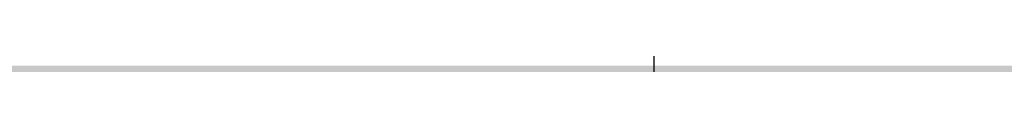
# Model space of a CAD drawing. Units: inches. Extents: x 2083 to 3317, y 1141 to 2115.
# Tile 60 of 256: x 2237.106 to 2238.294, y 1477.763 to 1477.764. Entities that reach past the tile are written whole.
import ezdxf

# ---------------------------------------------------------------- set-up
doc = ezdxf.new("R2010")
doc.units = ezdxf.units.IN
doc.layers.add('A-ANNO-DIMS', color=2, linetype='Continuous', lineweight=18)
doc.layers.add('A-WALL-PATT', color=251, linetype='Continuous', lineweight=13, true_color=0x636466)
doc.styles.get("Standard").update_dxf_attribs({"font": 'arial.ttf'})
doc.dimstyles.new('ISO-25', dxfattribs={"dimtxt": 12, "dimasz": 12, "dimexe": 1.25, "dimexo": 0.625, "dimtad": 1, "dimlunit": 3, "dimtxsty": 'Standard', "dimcen": 2.5, "dimadec": 0, "dimazin": 0, "dimtfac": 1, "dimtmove": 0, "dimatfit": 3, "dimfxl": 1, "dimarcsym": 0})

# ---------------------------------------------------------------- blocks, each defined once
blk = doc.blocks.new('*D30')
at = {"layer": 'A-ANNO-DIMS', "color": 0, "lineweight": -2, "transparency": 16777216}
for p, q in [((2240.0179, 1445.2738), (2240.0179, 1448.0455)), ((2254.3293, 1445.2738), (2254.3293, 1448.0455)), ((2228.0179, 1446.7955), (2216.0179, 1446.7955)), ((2240.0179, 1446.7955), (2254.3293, 1446.7955)), ((2266.3293, 1446.7955), (2413.7649, 1446.7955))]:
    blk.add_line(p, q, dxfattribs=at)
at = {"layer": 'A-ANNO-DIMS', "color": 0, "transparency": 16777216}
for points in [[(2228.0179, 1448.7955), (2228.0179, 1444.7955), (2240.0179, 1446.7955)], [(2266.3293, 1448.7955), (2266.3293, 1444.7955), (2254.3293, 1446.7955)]]:
    blk.add_solid(points, dxfattribs=at)
at = {"layer": 'Defpoints', "color": 0, "transparency": 16777216}
for p in [(2254.3293, 1446.7955), (2240.0179, 1444.6488), (2254.3293, 1444.6488)]:
    blk.add_point(p, dxfattribs=at)
at = {"layer": 'A-ANNO-DIMS', "color": 0, "transparency": 16777216, "insert": (2346.0471, 1453.6252), "char_height": 12, "attachment_point": 5}
blk.add_mtext('WC 1\'-2 1/2" TYP.', dxfattribs=at)
blk = doc.blocks.new('*D31')
at = {"layer": 'A-ANNO-DIMS', "color": 0, "lineweight": -2, "transparency": 16777216}
for p, q in [((2237.8711, 1456.6488), (2237.8711, 1541.9152)), ((2239.3929, 1444.6488), (2236.6211, 1444.6488)), ((2237.8711, 1431.5475), (2237.8711, 1444.6488)), ((2239.3929, 1431.5475), (2236.6211, 1431.5475)), ((2237.8711, 1419.5475), (2237.8711, 1407.5475))]:
    blk.add_line(p, q, dxfattribs=at)
at = {"layer": 'A-ANNO-DIMS', "color": 0, "transparency": 16777216}
for points in [[(2235.8711, 1456.6488), (2239.8711, 1456.6488), (2237.8711, 1444.6488)], [(2235.8711, 1419.5475), (2239.8711, 1419.5475), (2237.8711, 1431.5475)]]:
    blk.add_solid(points, dxfattribs=at)
at = {"layer": 'Defpoints', "color": 0, "transparency": 16777216}
for p in [(2237.8711, 1444.6488), (2240.0179, 1444.6488), (2240.0179, 1431.5475)]:
    blk.add_point(p, dxfattribs=at)
at = {"layer": 'A-ANNO-DIMS', "color": 0, "transparency": 16777216, "insert": (2231.2175, 1505.282), "char_height": 12, "attachment_point": 5, "rotation": 90}
blk.add_mtext('1\'-1" TYP.', dxfattribs=at)
blk = doc.blocks.new('*D45')
at = {"layer": 'A-ANNO-DIMS', "color": 0, "lineweight": -2, "transparency": 16777216}
for p, q in [((2235.9598, 1478.3864), (2235.9598, 1531.3614)), ((2418.9598, 1478.3864), (2418.9598, 1531.3614)), ((2247.9598, 1530.1114), (2406.9598, 1530.1114))]:
    blk.add_line(p, q, dxfattribs=at)
at = {"layer": 'A-ANNO-DIMS', "color": 0, "transparency": 16777216}
for points in [[(2247.9598, 1532.1114), (2247.9598, 1528.1114), (2235.9598, 1530.1114)], [(2406.9598, 1532.1114), (2406.9598, 1528.1114), (2418.9598, 1530.1114)]]:
    blk.add_solid(points, dxfattribs=at)
at = {"layer": 'Defpoints', "color": 0, "transparency": 16777216}
for p in [(2418.9598, 1530.1114), (2235.9598, 1477.7614), (2418.9598, 1477.7614)]:
    blk.add_point(p, dxfattribs=at)
at = {"layer": 'A-ANNO-DIMS', "color": 0, "transparency": 16777216, "insert": (2327.4598, 1536.8673), "char_height": 12, "attachment_point": 5}
blk.add_mtext('15\'-3"', dxfattribs=at)
blk = doc.blocks.new('*D62')
at = {"layer": 'A-ANNO-DIMS', "color": 0, "lineweight": -2, "transparency": 16777216}
for p, q in [((2235.9598, 1469.3864), (2235.9598, 1522.3614)), ((2379.9598, 1469.3864), (2379.9598, 1522.3614)), ((2247.9598, 1521.1114), (2367.9598, 1521.1114))]:
    blk.add_line(p, q, dxfattribs=at)
at = {"layer": 'A-ANNO-DIMS', "color": 0, "transparency": 16777216}
for points in [[(2247.9598, 1523.1114), (2247.9598, 1519.1114), (2235.9598, 1521.1114)], [(2367.9598, 1523.1114), (2367.9598, 1519.1114), (2379.9598, 1521.1114)]]:
    blk.add_solid(points, dxfattribs=at)
at = {"layer": 'Defpoints', "color": 0, "transparency": 16777216}
for p in [(2379.9598, 1521.1114), (2235.9598, 1468.7614), (2379.9598, 1468.7614)]:
    blk.add_point(p, dxfattribs=at)
at = {"layer": 'A-ANNO-DIMS', "color": 0, "transparency": 16777216, "insert": (2307.9598, 1527.8632), "char_height": 12, "attachment_point": 5}
blk.add_mtext('12\'-0"', dxfattribs=at)

msp = doc.modelspace()

# ---------------------------------------------------------------- hatches: boundary and pattern name
at = {"layer": 'A-WALL-PATT'}
h = msp.add_hatch(color=256, dxfattribs=at)
h.dxf.hatch_style = 1
h.paths.add_polyline_path([(3126.9598, 2020.7614), (2748.9598, 2020.7614), (2604.9598, 2020.7614), (2226.9598, 2020.7614), (2226.9598, 1702.7614), (2466.9598, 1702.7614), (2466.9598, 1582.7614), (2418.9598, 1582.7614), (2418.9598, 1477.7614), (2226.9598, 1477.7614), (2226.9598, 1263.2614), (2544.9598, 1263.2614), (2544.9598, 1411.7614), (2604.9598, 1411.7614), (2685.9598, 1411.7614), (2685.9598, 1420.7614), (2604.9598, 1420.7614), (2604.9598, 1573.7614), (2604.9598, 1702.7614), (2604.9598, 2011.7614), (2748.9598, 2011.7614), (2748.9598, 1702.7614), (2862.9598, 1702.7614), (2862.9598, 1621.7614), (2871.9598, 1621.7614), (2871.9598, 1702.7614), (2883.9598, 1702.7614), (2883.9598, 1706.9395, -0.026459), (2883.9598, 1711.7614), (2757.9598, 1711.7614), (2757.9598, 1807.7614), (2787.9598, 1807.7614), (2787.9598, 1812.2614), (2757.9598, 1812.2614), (2757.9598, 2011.7614), (2877.9598, 2011.7614), (2877.9598, 1812.2614), (2847.9598, 1812.2614), (2847.9598, 1807.7614), (2889.8357, 1807.7614), (2889.8357, 1812.2614), (2882.4598, 1812.2614), (2882.4598, 2011.7614), (3117.9598, 2011.7614), (3117.9598, 1812.2614), (2937.8357, 1812.2614), (2937.8357, 1807.7614), (2995.7098, 1807.7614), (2995.7098, 1796.1177), (3000.2098, 1796.1177), (3000.2098, 1807.7614), (3117.9598, 1807.7614), (3117.9598, 1711.7614), (3000.2098, 1711.7614), (3000.2098, 1760.1177), (2998.5727, 1760.1177, -0.020711), (2995.7098, 1760.1177), (2995.7098, 1711.7614), (2931.9598, 1711.7614), (2931.9598, 1702.7614), (3126.9598, 1702.7614)])
h.paths.add_polyline_path([(2471.4598, 2011.7614), (2471.4598, 1810.0114), (2462.7169, 1810.0114), (2462.7169, 1805.5114), (2505.9598, 1805.5114), (2505.9598, 1810.0114), (2475.9598, 1810.0114), (2475.9598, 2011.7614), (2595.9598, 2011.7614), (2595.9598, 1810.0114), (2565.9598, 1810.0114), (2565.9598, 1805.5114), (2595.9598, 1805.5114), (2595.9598, 1711.7614), (2235.9598, 1711.7614), (2235.9598, 1805.5114), (2353.7098, 1805.5114), (2353.7098, 1796.0542), (2358.2098, 1796.0542), (2358.2098, 1805.5114), (2414.7169, 1805.5114), (2414.7169, 1810.0114), (2235.9598, 1810.0114), (2235.9598, 2011.7614)], flags=16)
h.paths.add_polyline_path([(2270.2047, 1994.61), (2270.2047, 1970.61), (2246.2047, 1970.61), (2246.2047, 1994.61)], flags=0)
edge = h.paths.add_edge_path(flags=0)
edge.add_ellipse((2332.0274, 1899.7982), major_axis=(-3.043, 3.043), ratio=0.168252, start_angle=-161.3322, end_angle=-156.3071, ccw=False)
edge.add_ellipse((2333.082, 1898.7435), major_axis=(-1.0546, 1.0546), ratio=0.453532, start_angle=-123.371, end_angle=-94.1591)
edge = h.paths.add_edge_path(flags=0)
edge.add_ellipse((2332.0274, 1968.8763), major_axis=(3.043, 3.043), ratio=0.168252, start_angle=18.6678, end_angle=23.6929)
edge.add_spline(control_points=[(2332.9256, 1970.6911), (2332.2268, 1970.3361), (2330.8937, 1969.6589), (2328.4131, 1970.9321), (2327.2039, 1967.7487), (2324.7096, 1969.9556), (2322.5328, 1967.0124), (2320.0128, 1971.2958), (2317.6803, 1968.1578), (2316.0405, 1967.102), (2315.4269, 1966.8096)], knot_values=[0, 0, 0, 0, 2.267059, 4.324559, 6.685584, 8.878641, 11.121502, 14.300359, 17.755284, 19.732645, 19.732645, 19.732645, 19.732645], degree=3, periodic=0)
edge.add_ellipse((2332.0274, 1968.8763), major_axis=(3.043, 3.043), ratio=0.168252, start_angle=18.6678, end_angle=23.6929, ccw=False)
edge.add_ellipse((2333.082, 1969.9309), major_axis=(1.0546, 1.0546), ratio=0.453532, start_angle=56.629, end_angle=85.8409, ccw=False)
edge = h.paths.add_edge_path(flags=0)
edge.add_spline(control_points=[(2296.4283, 1967.9879), (2293.6278, 1965.3363), (2287.7036, 1959.7271), (2299.7439, 1949.9957), (2294.5326, 1935.6685), (2290.5732, 1920.6035), (2293.3941, 1909.9737), (2296.1854, 1904.9665)], knot_values=[0.099185, 0.099185, 0.099185, 0.099185, 0.345301, 0.619822, 0.982653, 1.386093, 1.810555, 1.810555, 1.810555, 1.810555], degree=3, periodic=0)
edge.add_spline(control_points=[(2296.1854, 1904.9665), (2297.3836, 1902.6193), (2298.001, 1901.9493), (2298.553, 1901.4682)], knot_values=[0.006246, 0.006246, 0.006246, 0.006246, 0.055476, 0.055476, 0.055476, 0.055476], degree=3, periodic=0)
edge.add_spline(control_points=[(2298.553, 1901.4682), (2297.2586, 1900.9232), (2295.2253, 1900.2321), (2293.0602, 1900.6142), (2292.1014, 1900.7884), (2292.0896, 1900.7906)], knot_values=[0.312835, 0.312835, 0.312835, 0.312835, 0.40178, 0.474987, 0.475903, 0.475903, 0.475903, 0.475903], degree=3, periodic=0)
edge.add_arc((2292.7936, 1904.6641), 3.937, 215.4209, 259.6982, ccw=False)
edge.add_spline(control_points=[(2289.5853, 1902.3823), (2289.4767, 1902.5351), (2289.3685, 1902.688), (2289.2609, 1902.8412)], knot_values=[0.102872, 0.102872, 0.102872, 0.102872, 0.116896, 0.116896, 0.116896, 0.116896], degree=3, periodic=0)
edge.add_spline(control_points=[(2289.2609, 1902.8412), (2288.6866, 1902.5502), (2287.64, 1902.0199), (2285.8813, 1901.874), (2283.853, 1901.5044), (2281.72, 1899.7105), (2278.467, 1899.4929), (2276.1571, 1901.8832), (2272.259, 1899.8041), (2267.7776, 1901.8432), (2262.2439, 1900.184), (2257.4149, 1901.7821), (2254.3184, 1900.7261), (2253.1783, 1900.3373)], knot_values=[0, 0, 0, 0, 1.907977, 3.477176, 5.261074, 7.972851, 11.680248, 13.717921, 16.939592, 22.789562, 27.502503, 33.595215, 37.145618, 37.145618, 37.145618, 37.145618], degree=3, periodic=0)
edge.add_line((2253.1783, 1900.3373), (2250.2442, 1902.8412))
edge.add_line((2250.2442, 1902.8412), (2250.2442, 1965.8333))
edge.add_line((2250.2442, 1965.8333), (2253.1783, 1968.3371))
edge.add_spline(control_points=[(2253.1783, 1968.3371), (2254.3184, 1967.9483), (2257.4149, 1966.8924), (2262.2439, 1968.4904), (2267.7776, 1966.8313), (2271.5267, 1968.5372), (2273.8759, 1967.8283), (2274.2067, 1967.7276)], knot_values=[0, 0, 0, 0, 0.09018, 0.244935, 0.364644, 0.513233, 0.537855, 0.537855, 0.537855, 0.537855], degree=3, periodic=0)
edge.add_arc((2274.3529, 1963.7933), 3.937, 72.0511, 92.1279, ccw=False)
edge.add_arc((2281.2969, 1985.23), 18.5963, 252.05113, 288.56572)
edge.add_arc((2292.3167, 1956.0289), 12.6461, 71.02679, 113.77822, ccw=False)
edge = h.paths.add_edge_path(flags=0)
edge.add_spline(control_points=[(2274.8994, 1951.8562), (2275.0662, 1951.6166), (2275.2327, 1951.3766), (2275.398, 1951.1359)], knot_values=[1.409916, 1.409916, 1.409916, 1.409916, 1.43159, 1.43159, 1.43159, 1.43159], degree=3, periodic=0)
edge.add_spline(control_points=[(2275.398, 1951.1359), (2275.7921, 1950.5619), (2276.1792, 1949.9838), (2276.5455, 1949.3971)], knot_values=[1.358238, 1.358238, 1.358238, 1.358238, 1.409916, 1.409916, 1.409916, 1.409916], degree=3, periodic=0)
edge.add_line((2276.5455, 1949.3971), (2277.4373, 1947.8622))
edge.add_spline(control_points=[(2277.4373, 1947.8622), (2276.3038, 1945.6731), (2274.6397, 1942.4269), (2274.6316, 1938.0939), (2272.7991, 1930.8515), (2274.3564, 1943.897), (2275.9477, 1947.9234), (2276.5455, 1949.3971)], knot_values=[0.005632, 0.005632, 0.005632, 0.005632, 0.186014, 0.266002, 0.357087, 0.59639, 0.739732, 0.739732, 0.739732, 0.739732], degree=3, periodic=0)
edge.add_spline(control_points=[(2276.5455, 1949.3971), (2276.1792, 1949.9838), (2275.7921, 1950.5619), (2275.398, 1951.1359)], knot_values=[1.358238, 1.358238, 1.358238, 1.358238, 1.409916, 1.409916, 1.409916, 1.409916], degree=3, periodic=0)
edge.add_spline(control_points=[(2275.398, 1951.1359), (2274.9425, 1950.0805), (2274.2078, 1948.0253), (2273.9346, 1944.8515), (2272.4685, 1937.6275), (2273.4662, 1945.6965), (2274.7006, 1951.0595), (2274.8994, 1951.8562)], knot_values=[0.104364, 0.104364, 0.104364, 0.104364, 0.189636, 0.269624, 0.36071, 0.600013, 0.644622, 0.644622, 0.644622, 0.644622], degree=3, periodic=0)
h.paths.add_polyline_path([(2269.1675, 1963.1276, -0.357527), (2268.1706, 1960.9764, -0.092561), (2268.1706, 1939.4363, -0.357527), (2269.1675, 1937.2851, -0.357527), (2267.0163, 1938.282, -0.164785), (2254.6856, 1938.282, -0.357527), (2252.5344, 1937.2851, -0.357527), (2253.5313, 1939.4363, -0.092561), (2253.5313, 1960.9764, -0.357527), (2252.5344, 1963.1276, -0.357527), (2254.6856, 1962.1307, -0.164785), (2267.0163, 1962.1307, -0.357527)], flags=0)
h.paths.add_polyline_path([(2248.8741, 1967.8018), (2248.8741, 1957.0277), (2249.4578, 1957.0277), (2249.4578, 1911.6468), (2248.8741, 1911.6468), (2248.8741, 1900.8727), (2246.5119, 1900.8727, 0.197327), (2244.1497, 1902.4569), (2244.1497, 1966.2176, 0.197327), (2246.5119, 1967.8018)], flags=0)
h.paths.add_polyline_path([(2269.1675, 1931.3893, -0.357527), (2268.1706, 1929.2381, -0.092561), (2268.1706, 1907.6981, -0.357527), (2269.1675, 1905.5469, -0.357527), (2267.0163, 1906.5438, -0.164785), (2254.6856, 1906.5438, -0.357527), (2252.5344, 1905.5469, -0.357527), (2253.5313, 1907.6981, -0.092561), (2253.5313, 1929.2381, -0.357527), (2252.5344, 1931.3893, -0.357527), (2254.6856, 1930.3925, -0.164785), (2267.0163, 1930.3925, -0.357527)], flags=0)
edge = h.paths.add_edge_path(flags=0)
edge.add_spline(control_points=[(2276.1969, 1906.7237), (2276.1681, 1909.0289), (2276.114, 1913.3719), (2270.5984, 1924.925), (2273.9052, 1919.0128), (2275.9217, 1916.2621), (2275.4746, 1912.4021), (2277.2579, 1910.3806), (2276.696, 1908.225), (2276.6462, 1906.813), (2276.6178, 1906.0084)], knot_values=[0, 0, 0, 0, 8.61026, 16.221274, 18.843057, 23.804898, 27.440828, 29.356102, 31.203478, 33.650687, 33.650687, 33.650687, 33.650687], degree=3, periodic=0)
edge.add_spline(control_points=[(2276.6178, 1906.0084), (2276.6233, 1905.6241), (2276.4977, 1904.6287), (2275.4418, 1903.8547), (2274.9373, 1903.0804), (2274.8591, 1902.8412)], knot_values=[0.156488, 0.156488, 0.156488, 0.156488, 0.184398, 0.231376, 0.250598, 0.250598, 0.250598, 0.250598], degree=3, periodic=0)
edge.add_line((2274.8591, 1902.8412), (2276.506, 1902.8412))
edge.add_spline(control_points=[(2276.506, 1902.8412), (2276.7883, 1903.0849), (2277.6651, 1904.1252), (2278.2495, 1904.3407), (2277.6539, 1908.5274), (2278.1557, 1906.2278), (2278.1005, 1905.2859), (2278.8467, 1904.069), (2277.8568, 1903.4149), (2277.8742, 1902.991), (2277.9036, 1902.8412)], knot_values=[0.059574, 0.059574, 0.059574, 0.059574, 0.080753, 0.103741, 0.16972, 0.176036, 0.207137, 0.240474, 0.262341, 0.27366, 0.27366, 0.27366, 0.27366], degree=3, periodic=0)
edge.add_line((2277.9036, 1902.8412), (2280.0298, 1902.8412))
edge.add_spline(control_points=[(2280.0298, 1902.8412), (2279.8882, 1903.0884), (2279.4993, 1903.9816), (2280.1523, 1905.9393), (2278.1036, 1909.6578), (2279.7624, 1907.1853), (2280.3279, 1904.8749), (2280.4851, 1903.4896), (2281.4633, 1903.2494), (2281.7583, 1902.9365), (2281.834, 1902.8412)], knot_values=[0.013856, 0.013856, 0.013856, 0.013856, 0.034874, 0.088867, 0.107879, 0.126738, 0.158714, 0.193757, 0.217487, 0.226722, 0.226722, 0.226722, 0.226722], degree=3, periodic=0)
edge.add_spline(control_points=[(2281.834, 1902.8412), (2281.7875, 1902.8267), (2281.647, 1902.783), (2281.3955, 1902.8595), (2281.0881, 1902.9852), (2280.7207, 1903.0609), (2280.3335, 1903.0257), (2280.1248, 1902.8989), (2280.0298, 1902.8412)], knot_values=[0, 0, 0, 0, 0.14413, 0.435517, 0.749276, 1.153046, 1.548371, 1.878348, 1.878348, 1.878348, 1.878348], degree=3, periodic=0)
edge.add_line((2280.0298, 1902.8412), (2277.9036, 1902.8412))
edge.add_spline(control_points=[(2277.9036, 1902.8412), (2277.8929, 1902.7959), (2277.8654, 1902.6796), (2277.6075, 1902.6875), (2277.2741, 1902.8007), (2276.8379, 1902.6198), (2276.5838, 1902.7893), (2276.506, 1902.8412)], knot_values=[0, 0, 0, 0, 0.127189, 0.326199, 0.628009, 1.24357, 1.515331, 1.515331, 1.515331, 1.515331], degree=3, periodic=0)
edge.add_line((2276.506, 1902.8412), (2274.8591, 1902.8412))
edge.add_spline(control_points=[(2274.8591, 1902.8412), (2274.8144, 1902.8986), (2274.7251, 1903.0134), (2274.4935, 1903.119), (2274.2443, 1902.9605), (2273.9371, 1903.1849), (2273.614, 1902.9831), (2273.4083, 1902.883), (2273.3223, 1902.8412)], knot_values=[0, 0, 0, 0, 0.21843, 0.436957, 0.687977, 0.990379, 1.398396, 1.69185, 1.69185, 1.69185, 1.69185], degree=3, periodic=0)
edge.add_spline(control_points=[(2273.3223, 1902.8412), (2273.6167, 1903.4457), (2274.274, 1904.5383), (2276.0272, 1904.5737), (2276.207, 1906.5836), (2276.1969, 1906.7237)], knot_values=[0.012227, 0.012227, 0.012227, 0.012227, 0.059472, 0.106218, 0.134458, 0.134458, 0.134458, 0.134458], degree=3, periodic=0)
h.paths.add_polyline_path([(2270.7761, 1897.7898), (2270.7761, 1873.7898), (2246.7761, 1873.7898), (2246.7761, 1897.7898)], flags=0)
h.paths.add_polyline_path([(2353.7098, 1760.0051), (2353.7098, 1760.0542), (2358.2098, 1760.0542, -0.033729)], flags=0)
h.paths.add_polyline_path([(2321.8191, 1737.5292), (2341.9953, 1737.5292, -0.414214), (2343.2033, 1736.3212), (2343.2033, 1721.0206, -0.414214), (2341.9953, 1719.8127), (2321.8191, 1719.8127, -0.414214), (2320.6112, 1721.0206), (2320.6112, 1736.3212, -0.414214)], flags=0)
h.paths.add_polyline_path([(2324.235, 1736.3212), (2339.5794, 1736.3212, -0.414214), (2341.9953, 1733.9053), (2341.9953, 1725.4497, -0.414214), (2339.5794, 1723.0338), (2333.6806, 1723.0338), (2333.8453, 1722.0455, -0.870646), (2335.4254, 1721.8259, -0.767327), (2333.9227, 1721.4232), (2331.291, 1721.4232, -0.767327), (2329.7883, 1721.8259, -0.870646), (2331.3684, 1722.0455), (2331.5331, 1723.0338), (2324.235, 1723.0338, -0.414214), (2321.8191, 1725.4497), (2321.8191, 1733.9053, -0.414214)], flags=0)
h.paths.add_polyline_path([(2570.4838, 1928.6154), (2589.6838, 1928.6154), (2590.1688, 1928.6154), (2590.1688, 1904.9934), (2570.4838, 1904.9934)], flags=0)
h.paths.add_polyline_path([(2574.4473, 1927.2638, -1), (2572.8288, 1927.2638, -1)], flags=0)
h.paths.add_polyline_path([(2573.0899, 1926.9409), (2573.925, 1927.776), (2574.1477, 1927.5533), (2573.3126, 1926.7182)], flags=0)
h.paths.add_polyline_path([(2578.7791, 1919.7296, -1), (2571.5917, 1919.7296, -1)], flags=0)
h.paths.add_polyline_path([(2578.3854, 1919.7296, -1), (2571.9854, 1919.7296, -1)], flags=0)
h.paths.add_polyline_path([(2331.5958, 1729.4762, -1), (2333.618, 1729.4762, -1)], flags=0)
h.paths.add_polyline_path([(2578.0342, 1927.2638, -1), (2576.4157, 1927.2638, -1)], flags=0)
h.paths.add_polyline_path([(2576.6889, 1927.5311), (2576.9116, 1927.7538), (2577.7467, 1926.9186), (2577.524, 1926.6959)], flags=0)
h.paths.add_polyline_path([(2578.1391, 1909.8595, -1), (2572.2317, 1909.8595, -1)], flags=0)
h.paths.add_polyline_path([(2577.7454, 1909.8595, -1), (2572.6254, 1909.8595, -1)], flags=0)
h.paths.add_polyline_path([(2583.7977, 1927.2638, -1), (2582.1792, 1927.2638, -1)], flags=0)
h.paths.add_polyline_path([(2582.7186, 1927.7538), (2583.5538, 1926.9186), (2583.3311, 1926.6959), (2582.4959, 1927.5311)], flags=0)
h.paths.add_polyline_path([(2582.4959, 1927.5311), (2582.7186, 1927.7538), (2583.5538, 1926.9186), (2583.3311, 1926.6959)], flags=0)
h.paths.add_polyline_path([(2587.7391, 1920.5296, -1), (2581.8317, 1920.5296, -1)], flags=0)
h.paths.add_polyline_path([(2587.3454, 1920.5296, -1), (2582.2254, 1920.5296, -1)], flags=0)
h.paths.add_polyline_path([(2587.3846, 1927.2638, -1), (2585.7661, 1927.2638, -1)], flags=0)
h.paths.add_polyline_path([(2586.082, 1926.9802), (2586.9172, 1927.8154), (2587.1399, 1927.5927), (2586.3047, 1926.7575)], flags=0)
h.paths.add_polyline_path([(2588.3791, 1910.6595, -1), (2581.1917, 1910.6595, -1)], flags=0)
h.paths.add_polyline_path([(2587.9854, 1910.6595, -1), (2581.5854, 1910.6595, -1)], flags=0)
h.paths.add_polyline_path([(2417.1677, 1729.4779), (2437.3439, 1729.4779, -0.414214), (2438.5519, 1728.2699), (2438.5519, 1712.9693, -0.414214), (2437.3439, 1711.7614), (2417.1677, 1711.7614, -0.414214), (2415.9598, 1712.9693), (2415.9598, 1728.2699, -0.414214)], flags=0)
h.paths.add_polyline_path([(2419.5836, 1728.2699), (2434.928, 1728.2699, -0.414214), (2437.3439, 1725.8541), (2437.3439, 1717.3984, -0.414214), (2434.928, 1714.9825), (2429.0292, 1714.9825), (2429.1939, 1713.9942, -0.870646), (2430.774, 1713.7746, -0.767327), (2429.2713, 1713.372), (2426.6396, 1713.372, -0.767327), (2425.1369, 1713.7746, -0.870646), (2426.717, 1713.9942), (2426.8817, 1714.9825), (2419.5836, 1714.9825, -0.414214), (2417.1677, 1717.3984), (2417.1677, 1725.8541, -0.414214)], flags=0)
h.paths.add_polyline_path([(2419.5836, 1728.2699), (2434.928, 1728.2699, -0.414214), (2437.3439, 1725.8541), (2437.3439, 1717.3984, -0.414214), (2434.928, 1714.9825), (2429.0292, 1714.9825), (2428.3581, 1719.009), (2427.5528, 1719.009), (2426.8817, 1714.9825), (2419.5836, 1714.9825, -0.414214), (2417.1677, 1717.3984), (2417.1677, 1725.8541, -0.414214)], flags=0)
h.paths.add_polyline_path([(2426.9444, 1721.4249, -1), (2428.9666, 1721.4249, -1)], flags=0)
h.paths.add_polyline_path([(2475.9598, 1702.7614), (2595.9598, 1702.7614), (2595.9598, 1582.7614), (2475.9598, 1582.7614)], flags=16)
h.paths.add_polyline_path([(2427.9598, 1573.7614), (2595.9598, 1573.7614), (2595.9598, 1468.7614), (2595.9598, 1420.7614), (2384.4598, 1420.7614), (2384.4598, 1468.7614), (2427.9598, 1468.7614)], flags=16)
h.paths.add_polyline_path([(2379.9598, 1468.7614), (2379.9598, 1420.7614), (2235.9598, 1420.7614), (2235.9598, 1468.7614)], flags=16)
h.paths.add_polyline_path([(2317.816, 1466.6958), (2337.9922, 1466.6958, -0.414214), (2339.2002, 1465.4878), (2339.2002, 1450.1872, -0.414214), (2337.9922, 1448.9792), (2317.816, 1448.9792, -0.414214), (2316.6081, 1450.1872), (2316.6081, 1465.4878, -0.414214)], flags=0)
h.paths.add_polyline_path([(2320.2319, 1465.4878), (2335.5763, 1465.4878, -0.414214), (2337.9922, 1463.0719), (2337.9922, 1454.6163, -0.414214), (2335.5763, 1452.2004), (2329.6775, 1452.2004), (2329.8422, 1451.212, -0.870646), (2331.4223, 1450.9925, -0.767327), (2329.9196, 1450.5898), (2327.2879, 1450.5898, -0.767327), (2325.7852, 1450.9925, -0.870646), (2327.3653, 1451.212), (2327.53, 1452.2004), (2320.2319, 1452.2004, -0.414214), (2317.816, 1454.6163), (2317.816, 1463.0719, -0.414214)], flags=0)
h.paths.add_polyline_path([(2320.2319, 1465.4878), (2335.5763, 1465.4878, -0.414214), (2337.9922, 1463.0719), (2337.9922, 1454.6163, -0.414214), (2335.5763, 1452.2004), (2329.6775, 1452.2004), (2329.0064, 1456.2269), (2328.2011, 1456.2269), (2327.53, 1452.2004), (2320.2319, 1452.2004, -0.414214), (2317.816, 1454.6163), (2317.816, 1463.0719, -0.414214)], flags=0)
h.paths.add_polyline_path([(2327.5926, 1458.6428, -1), (2329.6148, 1458.6428, -1)], flags=0)
h.paths.add_polyline_path([(2244.4117, 1433.3405), (2241.9209, 1433.3405, -0.414214), (2240.0179, 1435.2435), (2240.0179, 1440.9528, -0.414211), (2241.9209, 1442.8559), (2244.4117, 1442.8559, -1.976472)], flags=0)
h.paths.add_polyline_path([(2245.3569, 1434.3975, -0.414214), (2245.3569, 1441.7988, -2.144098)], flags=0)
h.paths.add_polyline_path([(2535.9598, 1416.2614), (2535.9598, 1272.2614), (2235.9598, 1272.2614), (2235.9598, 1416.2614)], flags=16)
h.paths.add_polyline_path([(2260.1196, 1384.2928), (2260.1196, 1362.0386), (2237.8654, 1362.0386), (2237.8654, 1384.2928)], flags=0)
edge = h.paths.add_edge_path(flags=0)
edge.add_line((2318.2518, 1362.0933), (2318.1458, 1362.001))
edge.add_ellipse((2317.4451, 1360.431), major_axis=(2.8216, 2.8216), ratio=0.168252, start_angle=18.6678, end_angle=20.9481, ccw=False)
edge.add_ellipse((2318.423, 1361.409), major_axis=(0.9779, 0.9779), ratio=0.453532, start_angle=56.629, end_angle=70.2262, ccw=False)
edge = h.paths.add_edge_path(flags=0)
edge.add_line((2319.1074, 1295.5711), (2319.015, 1295.6771))
edge.add_ellipse((2317.4451, 1296.3778), major_axis=(-2.8216, 2.8216), ratio=0.168252, start_angle=-161.3322, end_angle=-159.0519, ccw=False)
edge.add_ellipse((2318.423, 1295.3999), major_axis=(-0.9779, 0.9779), ratio=0.453532, start_angle=-123.371, end_angle=-109.7738)
edge = h.paths.add_edge_path(flags=0)
edge.add_spline(control_points=[(2284.2103, 1301.1702), (2284.5807, 1300.4447), (2284.8912, 1299.892), (2285.1596, 1299.461)], knot_values=[0.039066, 0.039066, 0.039066, 0.039066, 0.055476, 0.055476, 0.055476, 0.055476], degree=3, periodic=0)
edge.add_line((2285.1596, 1299.461), (2284.2103, 1301.1702))
edge = h.paths.add_edge_path(flags=0)
edge.add_line((2280.4125, 1297.298), (2283.37, 1297.0361))
edge.add_line((2283.37, 1297.0361), (2286.4057, 1297.9263))
edge.add_spline(control_points=[(2286.4057, 1297.9263), (2285.3055, 1297.4631), (2284.3448, 1297.1292), (2283.37, 1297.0361)], knot_values=[0.394369, 0.394369, 0.394369, 0.394369, 0.475903, 0.475903, 0.475903, 0.475903], degree=3, periodic=0)
edge.add_spline(control_points=[(2283.37, 1297.0361), (2283.2814, 1297.0277), (2282.3163, 1296.9573), (2281.3125, 1297.1345), (2280.4234, 1297.296), (2280.4125, 1297.298)], knot_values=[0.312835, 0.312835, 0.312835, 0.312835, 0.320246, 0.393453, 0.394369, 0.394369, 0.394369, 0.394369], degree=3, periodic=0)
edge = h.paths.add_edge_path(flags=0)
edge.add_line((2284.4356, 1359.6073), (2280.4463, 1355.328))
edge.add_line((2280.4463, 1355.328), (2279.58, 1351.0178))
edge.add_line((2279.58, 1351.0178), (2282.413, 1346.5804))
edge.add_spline(control_points=[(2282.413, 1346.5804), (2283.1533, 1345.5892), (2284.2529, 1344.0289), (2284.801, 1342.3872), (2284.9352, 1341.8055)], knot_values=[1.240098, 1.240098, 1.240098, 1.240098, 1.332892, 1.382712, 1.382712, 1.382712, 1.382712], degree=3, periodic=0)
edge.add_spline(control_points=[(2284.9352, 1341.8055), (2285.3191, 1340.1406), (2285.233, 1338.4092), (2284.9099, 1336.6541)], knot_values=[1.097484, 1.097484, 1.097484, 1.097484, 1.240098, 1.240098, 1.240098, 1.240098], degree=3, periodic=0)
edge.add_spline(control_points=[(2284.9099, 1336.6541), (2284.5868, 1334.899), (2284.0267, 1333.1203), (2283.4626, 1331.3606)], knot_values=[0.95487, 0.95487, 0.95487, 0.95487, 1.097484, 1.097484, 1.097484, 1.097484], degree=3, periodic=0)
edge.add_line((2283.4626, 1331.3606), (2281.8904, 1326.1534))
edge.add_line((2281.8904, 1326.1534), (2280.7563, 1321.0561))
edge.add_line((2280.7563, 1321.0561), (2280.2992, 1316.002))
edge.add_line((2280.2992, 1316.002), (2280.7159, 1310.9501))
edge.add_line((2280.7159, 1310.9501), (2282.0281, 1305.9721))
edge.add_line((2282.0281, 1305.9721), (2284.2103, 1301.1702))
edge.add_spline(control_points=[(2284.2103, 1301.1702), (2283.3407, 1302.7302), (2282.6119, 1304.3365), (2282.0281, 1305.9721)], knot_values=[0.099185, 0.099185, 0.099185, 0.099185, 0.241799, 0.241799, 0.241799, 0.241799], degree=3, periodic=0)
edge.add_spline(control_points=[(2282.0281, 1305.9721), (2281.4443, 1307.6078), (2281.0055, 1309.2728), (2280.7159, 1310.9501)], knot_values=[0.241799, 0.241799, 0.241799, 0.241799, 0.384413, 0.384413, 0.384413, 0.384413], degree=3, periodic=0)
edge.add_spline(control_points=[(2280.7159, 1310.9501), (2280.4332, 1312.5876), (2280.2894, 1314.277), (2280.2989, 1315.962), (2280.2992, 1316.002)], knot_values=[0.384413, 0.384413, 0.384413, 0.384413, 0.523647, 0.527028, 0.527028, 0.527028, 0.527028], degree=3, periodic=0)
edge.add_spline(control_points=[(2280.2992, 1316.002), (2280.3123, 1317.687), (2280.4779, 1319.3679), (2280.7563, 1321.0561)], knot_values=[0.527028, 0.527028, 0.527028, 0.527028, 0.669642, 0.669642, 0.669642, 0.669642], degree=3, periodic=0)
edge.add_spline(control_points=[(2280.7563, 1321.0561), (2281.0346, 1322.7443), (2281.4259, 1324.4396), (2281.8904, 1326.1534)], knot_values=[0.669642, 0.669642, 0.669642, 0.669642, 0.812256, 0.812256, 0.812256, 0.812256], degree=3, periodic=0)
edge.add_spline(control_points=[(2281.8904, 1326.1534), (2282.2644, 1327.5333), (2282.7879, 1329.2618), (2283.3528, 1331.0178), (2283.4626, 1331.3606)], knot_values=[0.812256, 0.812256, 0.812256, 0.812256, 0.927087, 0.95487, 0.95487, 0.95487, 0.95487], degree=3, periodic=0)
edge.add_line((2283.4626, 1331.3606), (2284.9099, 1336.6541))
edge.add_line((2284.9099, 1336.6541), (2284.9352, 1341.8055))
edge.add_line((2284.9352, 1341.8055), (2282.413, 1346.5804))
edge.add_spline(control_points=[(2282.413, 1346.5804), (2281.2751, 1348.1038), (2280.0784, 1349.5703), (2279.58, 1351.0178)], knot_values=[1.382712, 1.382712, 1.382712, 1.382712, 1.525326, 1.525326, 1.525326, 1.525326], degree=3, periodic=0)
edge.add_spline(control_points=[(2279.58, 1351.0178), (2279.4433, 1351.4147), (2279.1363, 1352.8569), (2279.7352, 1354.2904), (2280.4463, 1355.328)], knot_values=[1.525326, 1.525326, 1.525326, 1.525326, 1.564439, 1.667941, 1.667941, 1.667941, 1.667941], degree=3, periodic=0)
edge.add_spline(control_points=[(2280.4463, 1355.328), (2281.4261, 1356.7578), (2282.9308, 1358.1826), (2284.4356, 1359.6073)], knot_values=[1.667941, 1.667941, 1.667941, 1.667941, 1.810555, 1.810555, 1.810555, 1.810555], degree=3, periodic=0)
edge.add_arc((2280.6231, 1348.5182), 11.7262, 71.02679, 113.77822)
edge.add_arc((2270.4049, 1375.5952), 17.2436, 252.05113, 288.56572, ccw=False)
edge.add_arc((2263.966, 1355.7178), 3.6506, 72.0511, 92.1279)
edge.add_arc((2263.966, 1355.7178), 3.6506, 92.1279, 177.9851)
edge.add_spline(control_points=[(2260.3176, 1355.8462), (2260.2604, 1354.2207), (2260.5513, 1350.1865), (2262.9993, 1346.7663), (2264.4727, 1344.649)], knot_values=[1.43159, 1.43159, 1.43159, 1.43159, 1.564144, 1.770695, 1.770695, 1.770695, 1.770695], degree=3, periodic=0)
edge.add_line((2264.4727, 1344.649), (2264.9356, 1343.9825))
edge.add_spline(control_points=[(2263.801, 1340.2481), (2263.8432, 1340.5141), (2264.0672, 1341.7565), (2264.5127, 1343.0025), (2264.935, 1343.9811)], knot_values=[0.53657, 0.53657, 0.53657, 0.53657, 0.559349, 0.644622, 0.644622, 0.644622, 0.644622], degree=3, periodic=0)
edge.add_spline(control_points=[(2264.935, 1343.9811), (2265.1178, 1343.715), (2265.2989, 1343.4479), (2265.4768, 1343.1794)], knot_values=[1.384077, 1.384077, 1.384077, 1.384077, 1.409916, 1.409916, 1.409916, 1.409916], degree=3, periodic=0)
edge.add_spline(control_points=[(2265.4768, 1343.1794), (2265.6546, 1342.9108), (2265.8293, 1342.6408), (2265.9991, 1342.3688)], knot_values=[1.358238, 1.358238, 1.358238, 1.358238, 1.384077, 1.384077, 1.384077, 1.384077], degree=3, periodic=0)
edge.add_line((2265.9991, 1342.3688), (2266.826, 1340.9455))
edge.add_spline(control_points=[(2266.826, 1340.9455), (2268.8944, 1337.0897), (2271.3982, 1325.843), (2270.5162, 1310.5686), (2275.9194, 1301.8606), (2277.7895, 1299.1994)], knot_values=[0.116896, 0.116896, 0.116896, 0.116896, 0.472987, 1.050969, 1.313793, 1.313793, 1.313793, 1.313793], degree=3, periodic=0)
edge.add_spline(control_points=[(2277.7895, 1299.1994), (2277.8394, 1299.1285), (2277.8894, 1299.0575), (2277.9396, 1298.9866)], knot_values=[0.109884, 0.109884, 0.109884, 0.109884, 0.116896, 0.116896, 0.116896, 0.116896], degree=3, periodic=0)
edge.add_line((2277.9396, 1298.9866), (2277.7888, 1299.1991))
edge.add_spline(control_points=[(2277.7888, 1299.1991), (2277.2566, 1298.9294), (2276.2864, 1298.4379), (2275.0394, 1298.3344), (2274.3833, 1298.2389), (2274.2153, 1298.2093)], knot_values=[33.12187, 33.12187, 33.12187, 33.12187, 35.029056, 36.598255, 37.144827, 37.144827, 37.144827, 37.144827], degree=3, periodic=0)
edge.add_line((2274.2153, 1298.2093), (2273.0731, 1297.893))
edge.add_spline(control_points=[(2273.0731, 1297.893), (2272.3229, 1297.5798), (2271.0392, 1296.5105), (2269.2484, 1296.2261), (2268.4231, 1296.3747)], knot_values=[26.532584, 26.532584, 26.532584, 26.532584, 29.198919, 31.839101, 31.839101, 31.839101, 31.839101], degree=3, periodic=0)
edge.add_line((2268.4231, 1296.3747), (2263.8785, 1297.4575))
edge.add_spline(control_points=[(2263.8785, 1297.4575), (2263.5561, 1297.3594), (2261.8603, 1296.8387), (2260.2388, 1297.2824), (2258.9335, 1297.5165)], knot_values=[15.919551, 15.919551, 15.919551, 15.919551, 16.939592, 21.226067, 21.226067, 21.226067, 21.226067], degree=3, periodic=0)
edge.add_line((2258.9335, 1297.5165), (2254.0552, 1297.329))
edge.add_spline(control_points=[(2254.0552, 1297.329), (2253.7555, 1297.2958), (2252.1137, 1297.1652), (2250.4619, 1297.5442), (2249.1297, 1297.6679)], knot_values=[5.306517, 5.306517, 5.306517, 5.306517, 6.276435, 10.613034, 10.613034, 10.613034, 10.613034], degree=3, periodic=0)
edge.add_line((2249.1297, 1297.6679), (2244.3316, 1296.8778))
edge.add_line((2244.3316, 1296.8778), (2241.611, 1299.1994))
edge.add_line((2241.611, 1299.1994), (2241.611, 1357.6094))
edge.add_line((2241.611, 1357.6094), (2244.3316, 1359.9311))
edge.add_line((2244.3316, 1359.9311), (2252.7288, 1359.5427))
edge.add_spline(control_points=[(2252.7288, 1359.5427), (2252.8709, 1359.5464), (2253.3057, 1359.5482), (2253.7398, 1359.5143), (2254.0317, 1359.4824)], knot_values=[0.233291, 0.233291, 0.233291, 0.233291, 0.244935, 0.268927, 0.268927, 0.268927, 0.268927], degree=3, periodic=0)
edge.add_line((2254.0317, 1359.4824), (2259.5872, 1359.4164))
edge.add_spline(control_points=[(2259.5872, 1359.4164), (2260.6771, 1359.6285), (2262.0732, 1359.897), (2263.5237, 1359.4593), (2263.8304, 1359.366)], knot_values=[0.422516, 0.422516, 0.422516, 0.422516, 0.513233, 0.537855, 0.537855, 0.537855, 0.537855], degree=3, periodic=0)
edge.add_arc((2263.966, 1355.7178), 3.6506, 72.0511, 92.1279, ccw=False)
edge.add_arc((2270.4049, 1375.5952), 17.2436, 252.05113, 288.56572)
edge.add_arc((2280.6231, 1348.5182), 11.7262, 71.02679, 113.77822, ccw=False)
h.paths.add_polyline_path([(2240.3405, 1359.4347), (2240.3405, 1349.4444), (2240.8818, 1349.4444), (2240.8818, 1307.3645), (2240.3405, 1307.3645), (2240.3405, 1297.3741), (2238.1502, 1297.3741, 0.197327), (2235.9598, 1298.8431), (2235.9598, 1357.9657, 0.197327), (2238.1502, 1359.4347)], flags=0)
h.paths.add_polyline_path([(2259.1578, 1355.1005, -0.357527), (2258.2334, 1353.1058, -0.092561), (2258.2334, 1333.1326, -0.357527), (2259.1578, 1331.1379, -0.357527), (2257.1631, 1332.0622, -0.164785), (2245.7293, 1332.0622, -0.357527), (2243.7346, 1331.1379, -0.357527), (2244.6589, 1333.1326, -0.092561), (2244.6589, 1353.1058, -0.357527), (2243.7346, 1355.1005, -0.357527), (2245.7293, 1354.1761, -0.164785), (2257.1631, 1354.1761, -0.357527)], flags=0)
edge = h.paths.add_edge_path(flags=0)
edge.add_line((2265.9991, 1342.3688), (2266.826, 1340.9455))
edge.add_line((2266.826, 1340.9455), (2265.3076, 1337.8141))
edge.add_line((2265.3076, 1337.8141), (2264.3582, 1334.6529))
edge.add_line((2264.3582, 1334.6529), (2264.262, 1333.7997))
edge.add_spline(control_points=[(2264.262, 1333.7997), (2264.2084, 1333.1871), (2264.1621, 1332.3655), (2264.0071, 1331.4139), (2263.969, 1331.2018)], knot_values=[0.464444, 0.464444, 0.464444, 0.464444, 0.516691, 0.531608, 0.531608, 0.531608, 0.531608], degree=3, periodic=0)
edge.add_spline(control_points=[(2263.969, 1331.2018), (2263.7745, 1330.1189), (2263.4244, 1328.7908), (2263.2574, 1328.5307), (2263.234, 1328.5146)], knot_values=[0.372682, 0.372682, 0.372682, 0.372682, 0.44885, 0.464444, 0.464444, 0.464444, 0.464444], degree=3, periodic=0)
edge.add_spline(control_points=[(2263.234, 1328.5146), (2263.0964, 1328.4202), (2263.1312, 1329.3015), (2263.275, 1330.6157)], knot_values=[0.280919, 0.280919, 0.280919, 0.280919, 0.372682, 0.372682, 0.372682, 0.372682], degree=3, periodic=0)
edge.add_spline(control_points=[(2263.275, 1330.6157), (2263.4187, 1331.93), (2263.6715, 1333.6773), (2263.9699, 1335.315)], knot_values=[0.189157, 0.189157, 0.189157, 0.189157, 0.280919, 0.280919, 0.280919, 0.280919], degree=3, periodic=0)
edge.add_spline(control_points=[(2263.9699, 1335.315), (2264.1005, 1336.0322), (2264.4188, 1337.6219), (2264.7548, 1338.8644), (2264.9474, 1339.4911)], knot_values=[0.097394, 0.097394, 0.097394, 0.097394, 0.137578, 0.189157, 0.189157, 0.189157, 0.189157], degree=3, periodic=0)
edge.add_spline(control_points=[(2264.9474, 1339.4911), (2265.29, 1340.6061), (2265.6442, 1341.494), (2265.9991, 1342.3688)], knot_values=[0.005632, 0.005632, 0.005632, 0.005632, 0.097394, 0.097394, 0.097394, 0.097394], degree=3, periodic=0)
h.paths.add_polyline_path([(2259.1578, 1325.671, -0.357527), (2258.2334, 1323.6763, -0.092561), (2258.2334, 1303.7031, -0.357527), (2259.1578, 1301.7084, -0.357527), (2257.1631, 1302.6327, -0.164785), (2245.7293, 1302.6327, -0.357527), (2243.7346, 1301.7084, -0.357527), (2244.6589, 1303.7031, -0.092561), (2244.6589, 1323.6763, -0.357527), (2243.7346, 1325.671, -0.357527), (2245.7293, 1324.7466, -0.164785), (2257.1631, 1324.7466, -0.357527)], flags=0)
edge = h.paths.add_edge_path(flags=0)
edge.add_spline(control_points=[(2261.7089, 1317.3114), (2261.6795, 1317.4176), (2261.7619, 1317.3885), (2262.4907, 1316.0899), (2262.9622, 1315.3009)], knot_values=[14.955861, 14.955861, 14.955861, 14.955861, 16.221274, 18.694826, 18.694826, 18.694826, 18.694826], degree=3, periodic=0)
edge.add_spline(control_points=[(2262.9622, 1315.3009), (2262.9904, 1315.2536), (2263.7021, 1314.0674), (2264.349, 1313.1272), (2264.7301, 1312.1642)], knot_values=[18.694826, 18.694826, 18.694826, 18.694826, 18.843057, 22.433791, 22.433791, 22.433791, 22.433791], degree=3, periodic=0)
edge.add_spline(control_points=[(2264.7301, 1312.1642), (2264.8756, 1311.7964), (2265.1769, 1310.7698), (2265.1431, 1309.5593), (2265.2477, 1308.8242)], knot_values=[22.433791, 22.433791, 22.433791, 22.433791, 23.804898, 26.172756, 26.172756, 26.172756, 26.172756], degree=3, periodic=0)
edge.add_line((2265.2477, 1308.8242), (2265.8508, 1307.1719))
edge.add_spline(control_points=[(2265.8508, 1307.1719), (2266.065, 1306.8217), (2266.3844, 1306.3322), (2266.4244, 1305.7805), (2266.4204, 1305.6112)], knot_values=[28.062562, 28.062562, 28.062562, 28.062562, 29.356102, 29.911721, 29.911721, 29.911721, 29.911721], degree=3, periodic=0)
edge.add_spline(control_points=[(2266.4204, 1305.6112), (2266.4161, 1305.4326), (2266.394, 1305.25), (2266.3648, 1305.0659)], knot_values=[29.911721, 29.911721, 29.911721, 29.911721, 30.497837, 30.497837, 30.497837, 30.497837], degree=3, periodic=0)
edge.add_line((2266.3648, 1305.0659), (2266.0662, 1302.1363))
edge.add_spline(control_points=[(2266.0662, 1302.1363), (2266.0712, 1301.78), (2265.9981, 1301.2), (2265.6633, 1300.759), (2265.5089, 1300.5859)], knot_values=[0.156488, 0.156488, 0.156488, 0.156488, 0.184398, 0.203543, 0.203543, 0.203543, 0.203543], degree=3, periodic=0)
edge.add_line((2265.5089, 1300.5859), (2264.4353, 1299.1994))
edge.add_line((2264.4353, 1299.1994), (2265.9624, 1299.1994))
edge.add_line((2265.9624, 1299.1994), (2267.336, 1301.1753))
edge.add_line((2267.336, 1301.1753), (2267.3117, 1301.9862))
edge.add_spline(control_points=[(2267.3117, 1301.9862), (2267.2611, 1302.8624), (2267.1602, 1303.7371), (2267.2715, 1303.3259)], knot_values=[0.126229, 0.126229, 0.126229, 0.126229, 0.166617, 0.166617, 0.166617, 0.166617], degree=3, periodic=0)
edge.add_spline(control_points=[(2267.2715, 1303.3259), (2267.28, 1303.2943), (2267.3098, 1303.1754), (2267.3735, 1302.8836), (2267.4061, 1302.6828), (2267.4179, 1302.601)], knot_values=[0.166617, 0.166617, 0.166617, 0.166617, 0.16972, 0.176036, 0.180765, 0.180765, 0.180765, 0.180765], degree=3, periodic=0)
edge.add_spline(control_points=[(2267.7439, 1300.9875), (2267.6876, 1301.1509), (2267.4805, 1301.6567), (2267.4838, 1302.1448), (2267.4179, 1302.601)], knot_values=[0.180765, 0.180765, 0.180765, 0.180765, 0.193767, 0.220139, 0.220139, 0.220139, 0.220139], degree=3, periodic=0)
edge.add_line((2267.4179, 1302.601), (2267.7439, 1300.9875))
edge.add_spline(control_points=[(2267.7439, 1300.9875), (2267.832, 1300.7319), (2267.932, 1300.3099), (2267.5548, 1299.9745), (2267.4294, 1299.8292)], knot_values=[0.220139, 0.220139, 0.220139, 0.220139, 0.240474, 0.25489, 0.25489, 0.25489, 0.25489], degree=3, periodic=0)
edge.add_line((2267.4294, 1299.8292), (2267.2584, 1299.1994))
edge.add_line((2267.2584, 1299.1994), (2269.23, 1299.1994))
edge.add_spline(control_points=[(2269.23, 1299.1994), (2269.0987, 1299.4287), (2268.8428, 1300.0163), (2269.0116, 1300.9159), (2268.9468, 1301.6607)], knot_values=[0.013856, 0.013856, 0.013856, 0.013856, 0.034874, 0.067073, 0.067073, 0.067073, 0.067073], degree=3, periodic=0)
edge.add_line((2268.9468, 1301.6607), (2268.4316, 1303.6031))
edge.add_spline(control_points=[(2268.4316, 1303.6031), (2268.1756, 1304.1924), (2267.5962, 1305.2513), (2268.0407, 1304.6232), (2268.2514, 1304.2824)], knot_values=[0.090155, 0.090155, 0.090155, 0.090155, 0.107879, 0.120289, 0.120289, 0.120289, 0.120289], degree=3, periodic=0)
edge.add_spline(control_points=[(2268.2514, 1304.2824), (2268.3609, 1304.1053), (2269.0578, 1302.918), (2269.3827, 1301.5904), (2269.5214, 1300.7759), (2269.5752, 1300.5558)], knot_values=[0.120289, 0.120289, 0.120289, 0.120289, 0.126738, 0.158714, 0.173506, 0.173506, 0.173506, 0.173506], degree=3, periodic=0)
edge.add_line((2269.5752, 1300.5558), (2270.6858, 1299.4213))
edge.add_spline(control_points=[(2270.6858, 1299.4213), (2270.7672, 1299.3573), (2270.8379, 1299.2814), (2270.9029, 1299.1994)], knot_values=[0.21816, 0.21816, 0.21816, 0.21816, 0.226722, 0.226722, 0.226722, 0.226722], degree=3, periodic=0)
edge.add_line((2270.9372, 1299.1929), (2270.9029, 1299.1994))
edge.add_spline(control_points=[(2270.9029, 1299.1994), (2270.8598, 1299.186), (2270.7295, 1299.1455), (2270.4963, 1299.2164), (2270.2717, 1299.3083), (2270.121, 1299.348), (2270.0633, 1299.3596)], knot_values=[0.939174, 0.939174, 0.939174, 0.939174, 1.083304, 1.374691, 1.68845, 1.878348, 1.878348, 1.878348, 1.878348], degree=3, periodic=0)
edge.add_line((2270.0633, 1299.3596), (2269.23, 1299.1994))
edge.add_line((2269.23, 1299.1994), (2267.2584, 1299.1994))
edge.add_spline(control_points=[(2267.2584, 1299.1994), (2267.2484, 1299.1574), (2267.223, 1299.0497), (2266.9838, 1299.0569), (2266.8092, 1299.1162), (2266.6769, 1299.1091), (2266.6365, 1299.1048)], knot_values=[0.757665, 0.757665, 0.757665, 0.757665, 0.884854, 1.083864, 1.385675, 1.515331, 1.515331, 1.515331, 1.515331], degree=3, periodic=0)
edge.add_spline(control_points=[(2266.6365, 1299.1048), (2266.4852, 1299.0888), (2266.2358, 1299.0171), (2266.0346, 1299.1513), (2265.9624, 1299.1994)], knot_values=[0, 0, 0, 0, 0.485905, 0.757665, 0.757665, 0.757665, 0.757665], degree=3, periodic=0)
edge.add_line((2265.9624, 1299.1994), (2264.4353, 1299.1994))
edge.add_line((2264.4353, 1299.1994), (2263.8584, 1299.3671))
edge.add_spline(control_points=[(2263.8584, 1299.3671), (2263.8189, 1299.3709), (2263.7795, 1299.3857), (2263.7401, 1299.4015)], knot_values=[0.845925, 0.845925, 0.845925, 0.845925, 0.978627, 0.978627, 0.978627, 0.978627], degree=3, periodic=0)
edge.add_line((2263.7218, 1299.3964), (2263.0103, 1299.1994))
edge.add_spline(control_points=[(2263.0103, 1299.1994), (2263.2458, 1299.6829), (2263.506, 1300.1281), (2263.8735, 1300.408)], knot_values=[0.012227, 0.012227, 0.012227, 0.012227, 0.052971, 0.052971, 0.052971, 0.052971], degree=3, periodic=0)
edge.add_spline(control_points=[(2263.8735, 1300.408), (2263.9321, 1300.4527), (2264.0842, 1300.553), (2264.2552, 1300.6242), (2264.3597, 1300.6647)], knot_values=[0.052971, 0.052971, 0.052971, 0.052971, 0.059472, 0.069086, 0.069086, 0.069086, 0.069086], degree=3, periodic=0)
edge.add_line((2264.3597, 1300.6647), (2265.1419, 1301.0778))
edge.add_line((2265.1419, 1301.0778), (2265.6758, 1302.7996))
edge.add_line((2265.6758, 1302.7996), (2265.5407, 1305.7041))
edge.add_line((2265.5407, 1305.7041), (2264.8031, 1309.3277))
edge.add_line((2264.8031, 1309.3277), (2263.0405, 1314.0918))
edge.add_spline(control_points=[(2263.0405, 1314.0918), (2262.3836, 1315.6714), (2261.796, 1316.9977), (2261.7089, 1317.3114)], knot_values=[11.216896, 11.216896, 11.216896, 11.216896, 14.955861, 14.955861, 14.955861, 14.955861], degree=3, periodic=0)
h.paths.add_polyline_path([(2871.9598, 1416.2614), (2895.91, 1416.2614), (2895.91, 1420.7614), (2871.9598, 1420.7614), (2871.9598, 1501.7614), (2862.9598, 1501.7614), (2862.9598, 1420.7614), (2805.9598, 1420.7614), (2805.9598, 1411.7614), (2862.9598, 1411.7614), (2862.9598, 1263.2614), (3126.9598, 1263.2614), (3126.9598, 1411.7614), (3126.9598, 1486.7614), (2943.9598, 1486.7614), (2943.9598, 1477.7614), (2967.8603, 1477.7614), (2967.8603, 1420.7614), (2943.91, 1420.7614), (2943.91, 1416.2614), (3117.9598, 1416.2614), (3117.9598, 1420.7614), (2972.3603, 1420.7614), (2972.3603, 1477.7614), (3117.9598, 1477.7614), (3117.9598, 1420.7614), (3117.9598, 1272.2614), (2871.9598, 1272.2614)], flags=0)
h.paths.add_polyline_path([(2457.1256, 1485.9425), (2527.6027, 1485.9425), (2527.6027, 1537.6357), (2457.1256, 1537.6357)], flags=8)
h.paths.add_polyline_path([(2481.0051, 1609.9818), (2590.7658, 1609.9818), (2590.7658, 1682.0034), (2481.0051, 1682.0034)], flags=8)
h.paths.add_polyline_path([(2483.085, 1729.1268), (2553.562, 1729.1268), (2553.562, 1780.82), (2483.085, 1780.82)], flags=8)

# ---------------------------------------------------------------- dimensions: what is measured, and where the dimension line sits
at = {"layer": 'A-ANNO-DIMS'}
for base, p1, p2, picture, middle in [((2418.9598, 1530.1114), (2235.9598, 1477.7614), (2418.9598, 1477.7614), '*D45', (2327.4598, 1536.8673)), ((2379.9598, 1521.1114), (2235.9598, 1468.7614), (2379.9598, 1468.7614), '*D62', (2307.9598, 1527.8632))]:
    dim = msp.add_linear_dim(base=base, p1=p1, p2=p2, dimstyle='ISO-25', override={"dimdec": 1, "dimlfac": 1, "dimrnd": 0, "dimzin": 1, "dimdsep": 46, "dimlunit": 4, "dimfrac": 2}, dxfattribs=at)
    dim.commit()
    dim.dimension.update_dxf_attribs({"geometry": picture, "text_midpoint": middle})
dim = msp.add_linear_dim(base=(2237.8711, 1444.6488), p1=(2240.0179, 1431.5475), p2=(2240.0179, 1444.6488), angle=90, text='<> TYP.', dimstyle='ISO-25', override={"dimdec": 1, "dimlfac": 1, "dimrnd": 0, "dimzin": 1, "dimdsep": 46, "dimlunit": 4, "dimfrac": 2}, dxfattribs=at)
dim.commit()
dim.dimension.update_dxf_attribs({"geometry": '*D31', "text_midpoint": (2231.2175, 1505.282)})
dim = msp.add_linear_dim(base=(2254.3293, 1446.7955), p1=(2240.0179, 1444.6488), p2=(2254.3293, 1444.6488), text='WC <> TYP.', dimstyle='ISO-25', override={"dimdec": 1, "dimlfac": 1, "dimrnd": 0, "dimzin": 1, "dimdsep": 46, "dimlunit": 4, "dimfrac": 2}, dxfattribs=at)
dim.commit()
dim.dimension.update_dxf_attribs({"geometry": '*D30', "text_midpoint": (2346.0471, 1453.6252)})

doc.saveas('drawing.dxf')
